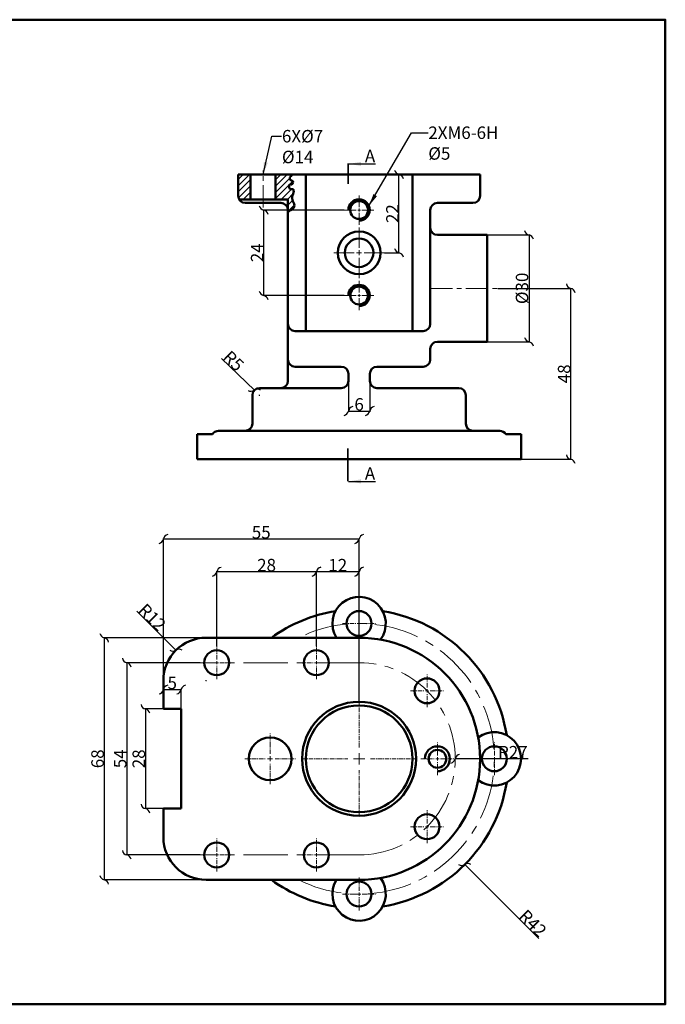
# Model space of a CAD drawing. Units: millimetres. Extents: x 10 to 373, y 9 to 285.
# Tile 3 of 3: x 191 to 373, y 9 to 285. Entities that reach past the tile are written whole.
import ezdxf

# ---------------------------------------------------------------- set-up
doc = ezdxf.new("R2010")
doc.units = ezdxf.units.MM
doc.header["$MEASUREMENT"] = 0
doc.linetypes.add('CENTER', pattern=[2, 1.25, -0.25, 0.25, -0.25])
for name, color, linetype, lineweight in [('M-CNTR', 1, 'CENTER', 18), ('M-DIMS', 2, 'Continuous', 25), ('M-HATC', 8, 'Continuous', 18), ('M-OUTL', 7, 'Continuous', 50), ('M-SECT', 7, 'Continuous', 35), ('M-TEXT', 7, 'Continuous', 25), ('M-TTLB', 7, 'Continuous', 50)]:
    doc.layers.add(name, color=color, linetype=linetype, lineweight=lineweight)
doc.styles.get("Standard").update_dxf_attribs({"font": 'arial.ttf'})
doc.dimstyles.get("Standard").update_dxf_attribs({"dimtxt": 3.5, "dimasz": 3.5, "dimexe": 0.18, "dimexo": 0.0625, "dimgap": 0.09, "dimtad": 1, "dimdec": 0, "dimzin": 0, "dimdsep": 46, "dimtxsty": 'Standard', "dimblk": 'INTEGRAL', "dimcen": 0.09, "dimclre": 251, "dimadec": 0, "dimazin": 0, "dimtfac": 1, "dimtdec": 0, "dimtofl": 0, "dimtmove": 0, "dimatfit": 3, "dimfxl": 1, "dimtolj": 1, "dimtzin": 0, "dimarcsym": 0})

# ---------------------------------------------------------------- blocks, each defined once
blk = doc.blocks.new('*U5')
at = {"layer": 'M-CNTR', "color": 0, "transparency": 16777216}
for p, q in [((0, 0.9), (0, 4.62)), ((-4.62, 0), (-0.9, 0)), ((0.9, 0), (4.62, 0)), ((0, -4.62), (0, -0.9))]:
    blk.add_line(p, q, dxfattribs=at)
at = {"layer": 'M-CNTR', "color": 0, "linetype": 'Continuous', "transparency": 16777216}
for p, q in [((-0.45, 0), (0.45, 0)), ((0, -0.45), (0, 0.45))]:
    blk.add_line(p, q, dxfattribs=at)
blk = doc.blocks.new('*U6')
at = {"layer": 'M-CNTR', "color": 0, "transparency": 16777216}
for p, q in [((0, 0.9), (0, 4.62)), ((-4.62, 0), (-0.9, 0)), ((0.9, 0), (4.62, 0)), ((0, -4.62), (0, -0.9))]:
    blk.add_line(p, q, dxfattribs=at)
at = {"layer": 'M-CNTR', "color": 0, "linetype": 'Continuous', "transparency": 16777216}
for p, q in [((-0.45, 0), (0.45, 0)), ((0, -0.45), (0, 0.45))]:
    blk.add_line(p, q, dxfattribs=at)
blk = doc.blocks.new('*U7')
at = {"layer": 'M-CNTR', "color": 0, "transparency": 16777216}
for p, q in [((0, 0.9), (0, 4.62)), ((-4.62, 0), (-0.9, 0)), ((0.9, 0), (4.62, 0)), ((0, -4.62), (0, -0.9))]:
    blk.add_line(p, q, dxfattribs=at)
at = {"layer": 'M-CNTR', "color": 0, "linetype": 'Continuous', "transparency": 16777216}
for p, q in [((-0.45, 0), (0.45, 0)), ((0, -0.45), (0, 0.45))]:
    blk.add_line(p, q, dxfattribs=at)
blk = doc.blocks.new('*U8')
at = {"layer": 'M-CNTR', "color": 0, "transparency": 16777216}
for p, q in [((0, 0.9), (0, 4.62)), ((-4.62, 0), (-0.9, 0)), ((0.9, 0), (4.62, 0)), ((0, -4.62), (0, -0.9))]:
    blk.add_line(p, q, dxfattribs=at)
at = {"layer": 'M-CNTR', "color": 0, "linetype": 'Continuous', "transparency": 16777216}
for p, q in [((-0.45, 0), (0.45, 0)), ((0, -0.45), (0, 0.45))]:
    blk.add_line(p, q, dxfattribs=at)
blk = doc.blocks.new('*U9')
at = {"layer": 'M-CNTR', "color": 0, "transparency": 16777216}
for p, q in [((0, 0.9), (0, 4.62)), ((-4.62, 0), (-0.9, 0)), ((0.9, 0), (4.62, 0)), ((0, -4.62), (0, -0.9))]:
    blk.add_line(p, q, dxfattribs=at)
at = {"layer": 'M-CNTR', "color": 0, "linetype": 'Continuous', "transparency": 16777216}
for p, q in [((-0.45, 0), (0.45, 0)), ((0, -0.45), (0, 0.45))]:
    blk.add_line(p, q, dxfattribs=at)
blk = doc.blocks.new('*U10')
at = {"layer": 'M-CNTR', "color": 0, "transparency": 16777216}
for p, q in [((0, 0.9), (0, 4.62)), ((-4.62, 0), (-0.9, 0)), ((0.9, 0), (4.62, 0)), ((0, -4.62), (0, -0.9))]:
    blk.add_line(p, q, dxfattribs=at)
at = {"layer": 'M-CNTR', "color": 0, "linetype": 'Continuous', "transparency": 16777216}
for p, q in [((-0.45, 0), (0.45, 0)), ((0, -0.45), (0, 0.45))]:
    blk.add_line(p, q, dxfattribs=at)
blk = doc.blocks.new('*U11')
at = {"layer": 'M-CNTR', "color": 0, "transparency": 16777216}
for p, q in [((0, 0.9), (0, 4.62)), ((-4.62, 0), (-0.9, 0)), ((0.9, 0), (4.62, 0)), ((0, -4.62), (0, -0.9))]:
    blk.add_line(p, q, dxfattribs=at)
at = {"layer": 'M-CNTR', "color": 0, "linetype": 'Continuous', "transparency": 16777216}
for p, q in [((-0.45, 0), (0.45, 0)), ((0, -0.45), (0, 0.45))]:
    blk.add_line(p, q, dxfattribs=at)
blk = doc.blocks.new('*U12')
at = {"layer": 'M-CNTR', "color": 0, "transparency": 16777216}
for p, q in [((0, 1.4), (0, 7.12)), ((-7.12, 0), (-1.4, 0)), ((1.4, 0), (7.12, 0)), ((0, -7.12), (0, -1.4))]:
    blk.add_line(p, q, dxfattribs=at)
at = {"layer": 'M-CNTR', "color": 0, "linetype": 'Continuous', "transparency": 16777216}
for p, q in [((-0.7, 0), (0.7, 0)), ((0, -0.7), (0, 0.7))]:
    blk.add_line(p, q, dxfattribs=at)
blk = doc.blocks.new('*U13')
at = {"layer": 'M-CNTR', "color": 0, "transparency": 16777216}
for p, q in [((0, 3.2), (0, 16.12)), ((-16.12, 0), (-3.2, 0)), ((3.2, 0), (16.12, 0)), ((0, -16.12), (0, -3.2))]:
    blk.add_line(p, q, dxfattribs=at)
at = {"layer": 'M-CNTR', "color": 0, "linetype": 'Continuous', "transparency": 16777216}
for p, q in [((-1.6, 0), (1.6, 0)), ((0, -1.6), (0, 1.6))]:
    blk.add_line(p, q, dxfattribs=at)
blk = doc.blocks.new('*U14')
at = {"layer": 'M-CNTR', "color": 0, "transparency": 16777216}
for p, q in [((0, 0.9), (0, 4.62)), ((-4.62, 0), (-0.9, 0)), ((0.9, 0), (4.62, 0)), ((0, -4.62), (0, -0.9))]:
    blk.add_line(p, q, dxfattribs=at)
at = {"layer": 'M-CNTR', "color": 0, "linetype": 'Continuous', "transparency": 16777216}
for p, q in [((-0.45, 0), (0.45, 0)), ((0, -0.45), (0, 0.45))]:
    blk.add_line(p, q, dxfattribs=at)
blk = doc.blocks.new('*U15')
at = {"layer": 'M-CNTR', "color": 0, "transparency": 16777216}
for p, q in [((0, 0.9), (0, 4.62)), ((-4.62, 0), (-0.9, 0)), ((0.9, 0), (4.62, 0)), ((0, -4.62), (0, -0.9))]:
    blk.add_line(p, q, dxfattribs=at)
at = {"layer": 'M-CNTR', "color": 0, "linetype": 'Continuous', "transparency": 16777216}
for p, q in [((-0.45, 0), (0.45, 0)), ((0, -0.45), (0, 0.45))]:
    blk.add_line(p, q, dxfattribs=at)
blk = doc.blocks.new('*U16')
at = {"layer": 'M-CNTR', "color": 0, "transparency": 16777216}
for p, q in [((0, 0.9), (0, 4.62)), ((-4.62, 0), (-0.9, 0)), ((0.9, 0), (4.62, 0)), ((0, -4.62), (0, -0.9))]:
    blk.add_line(p, q, dxfattribs=at)
at = {"layer": 'M-CNTR', "color": 0, "linetype": 'Continuous', "transparency": 16777216}
for p, q in [((-0.45, 0), (0.45, 0)), ((0, -0.45), (0, 0.45))]:
    blk.add_line(p, q, dxfattribs=at)
blk = doc.blocks.new('*U20')
at = {"layer": 'M-CNTR', "color": 0, "ltscale": 5, "transparency": 16777216}
for p, q in [((0, 0.8), (0, 4.12)), ((-4.12, 0), (-0.8, 0)), ((0.8, 0), (4.12, 0)), ((0, -4.12), (0, -0.8))]:
    blk.add_line(p, q, dxfattribs=at)
at = {"layer": 'M-CNTR', "color": 0, "linetype": 'Continuous', "ltscale": 5, "transparency": 16777216}
for p, q in [((-0.4, 0), (0.4, 0)), ((0, -0.4), (0, 0.4))]:
    blk.add_line(p, q, dxfattribs=at)
blk = doc.blocks.new('*U21')
at = {"layer": 'M-CNTR', "color": 0, "ltscale": 5, "transparency": 16777216}
for p, q in [((0, 1.4), (0, 7.12)), ((-7.12, 0), (-1.4, 0)), ((1.4, 0), (7.12, 0)), ((0, -7.12), (0, -1.4))]:
    blk.add_line(p, q, dxfattribs=at)
at = {"layer": 'M-CNTR', "color": 0, "linetype": 'Continuous', "ltscale": 5, "transparency": 16777216}
for p, q in [((-0.7, 0), (0.7, 0)), ((0, -0.7), (0, 0.7))]:
    blk.add_line(p, q, dxfattribs=at)
blk = doc.blocks.new('*U22')
at = {"layer": 'M-CNTR', "color": 0, "ltscale": 5, "transparency": 16777216}
for p, q in [((0, 0.8), (0, 4.12)), ((-4.12, 0), (-0.8, 0)), ((0.8, 0), (4.12, 0)), ((0, -4.12), (0, -0.8))]:
    blk.add_line(p, q, dxfattribs=at)
at = {"layer": 'M-CNTR', "color": 0, "linetype": 'Continuous', "ltscale": 5, "transparency": 16777216}
for p, q in [((-0.4, 0), (0.4, 0)), ((0, -0.4), (0, 0.4))]:
    blk.add_line(p, q, dxfattribs=at)
blk = doc.blocks.new('_Integral')
at = {"color": 0, "linetype": 'ByBlock', "lineweight": -2}
for centre, start, end in [((0.445, -0.091), 102, 168), ((-0.445, 0.091), 282, 348)]:
    blk.add_arc(centre, 0.454, start, end, dxfattribs=at)
blk = doc.blocks.new('*D45')
at = {"layer": 'Defpoints', "color": 0, "transparency": 16777216}
for p in [(259.92, 231.9), (282.61, 231.9), (282.61, 207.9)]:
    blk.add_point(p, dxfattribs=at)
at = {"layer": 'M-DIMS', "color": 0, "lineweight": -2, "transparency": 16777216}
for p, q in [((282.54, 231.9), (259.74, 231.9)), ((259.92, 207.9), (259.92, 231.9)), ((282.54, 207.9), (259.74, 207.9))]:
    blk.add_line(p, q, dxfattribs=at)
at = {"layer": 'M-DIMS', "color": 0, "lineweight": -2, "transparency": 16777216, "xscale": 3.5, "yscale": 3.5, "zscale": 3.5}
for p, rotation in [((259.92, 231.9), 90), ((259.92, 207.9), 270)]:
    blk.add_blockref('_Integral', p, dxfattribs=dict(at, rotation=rotation))
at = {"layer": 'M-DIMS', "color": 0, "transparency": 16777216, "insert": (258.07, 219.9), "char_height": 3.5, "attachment_point": 5, "rotation": 90}
blk.add_mtext('\\A1;24', dxfattribs=at)
blk = doc.blocks.new('*D46')
at = {"layer": 'Defpoints', "color": 0, "transparency": 16777216}
for p in [(297.94, 241.9), (298.06, 241.9), (293.85, 219.9)]:
    blk.add_point(p, dxfattribs=at)
at = {"layer": 'M-DIMS', "color": 0, "lineweight": -2, "transparency": 16777216}
for p, q in [((298, 241.9), (297.76, 241.9)), ((297.94, 219.9), (297.94, 241.9)), ((293.91, 219.9), (298.12, 219.9))]:
    blk.add_line(p, q, dxfattribs=at)
at = {"layer": 'M-DIMS', "color": 0, "lineweight": -2, "transparency": 16777216, "xscale": 3.5, "yscale": 3.5, "zscale": 3.5}
for p, rotation in [((297.94, 241.9), 90), ((297.94, 219.9), 270)]:
    blk.add_blockref('_Integral', p, dxfattribs=dict(at, rotation=rotation))
at = {"layer": 'M-DIMS', "color": 0, "transparency": 16777216, "insert": (296.09, 230.9), "char_height": 3.5, "attachment_point": 5, "rotation": 90}
blk.add_mtext('\\A1;22', dxfattribs=at)
blk = doc.blocks.new('*D47')
at = {"layer": 'Defpoints', "color": 0, "transparency": 16777216}
for p in [(322.73, 224.9), (322.73, 194.9), (334.48, 194.9)]:
    blk.add_point(p, dxfattribs=at)
at = {"layer": 'M-DIMS', "color": 0, "lineweight": -2, "transparency": 16777216}
for p, q in [((322.79, 224.9), (334.66, 224.9)), ((334.48, 224.9), (334.48, 194.9)), ((322.79, 194.9), (334.66, 194.9))]:
    blk.add_line(p, q, dxfattribs=at)
at = {"layer": 'M-DIMS', "color": 0, "lineweight": -2, "transparency": 16777216, "xscale": 3.5, "yscale": 3.5, "zscale": 3.5}
for p, rotation in [((334.48, 224.9), 90), ((334.48, 194.9), 270)]:
    blk.add_blockref('_Integral', p, dxfattribs=dict(at, rotation=rotation))
at = {"layer": 'M-DIMS', "color": 0, "transparency": 16777216, "insert": (332.51, 209.9), "char_height": 3.5, "attachment_point": 5, "rotation": 90}
blk.add_mtext('\\A1;%%C30', dxfattribs=at)
blk = doc.blocks.new('*D48')
at = {"layer": 'Defpoints', "color": 0, "transparency": 16777216}
for p in [(283.73, 183.9), (289.73, 183.9), (289.73, 175.44)]:
    blk.add_point(p, dxfattribs=at)
at = {"layer": 'M-DIMS', "color": 0, "lineweight": -2, "transparency": 16777216}
for p, q in [((283.73, 183.84), (283.73, 175.26)), ((289.73, 183.84), (289.73, 175.26)), ((283.73, 175.44), (289.73, 175.44))]:
    blk.add_line(p, q, dxfattribs=at)
at = {"layer": 'M-DIMS', "color": 0, "lineweight": -2, "transparency": 16777216, "xscale": 3.5, "yscale": 3.5, "zscale": 3.5, "rotation": 180}
blk.add_blockref('_Integral', (283.73, 175.44), dxfattribs=at)
at = {"layer": 'M-DIMS', "color": 0, "lineweight": -2, "transparency": 16777216, "xscale": 3.5, "yscale": 3.5, "zscale": 3.5}
blk.add_blockref('_Integral', (289.73, 175.44), dxfattribs=at)
at = {"layer": 'M-DIMS', "color": 0, "transparency": 16777216, "insert": (286.73, 177.32), "char_height": 3.5, "attachment_point": 5}
blk.add_mtext('\\A1;6', dxfattribs=at)
blk = doc.blocks.new('*D49')
at = {"layer": 'Defpoints', "color": 0, "transparency": 16777216}
for p in [(257.29, 181.29), (258.73, 179.9)]:
    blk.add_point(p, dxfattribs=at)
at = {"layer": 'M-DIMS', "color": 0, "lineweight": -2, "transparency": 16777216}
for p, q in [((248.05, 190.22), (257.29, 181.29)), ((258.64, 179.9), (258.82, 179.9)), ((258.73, 179.81), (258.73, 179.99))]:
    blk.add_line(p, q, dxfattribs=at)
at = {"layer": 'M-DIMS', "color": 0, "lineweight": -2, "transparency": 16777216, "xscale": 3.5, "yscale": 3.5, "zscale": 3.5, "rotation": 315.9975904098443}
blk.add_blockref('_Integral', (257.29, 181.29), dxfattribs=at)
at = {"layer": 'M-DIMS', "color": 0, "transparency": 16777216, "insert": (251.45, 189.53), "char_height": 3.5, "attachment_point": 5, "rotation": 315.9976}
blk.add_mtext('\\A1;R5', dxfattribs=at)
blk = doc.blocks.new('*D50')
at = {"layer": 'Defpoints', "color": 0, "transparency": 16777216}
for p in [(274.73, 130.31), (274.73, 109.38), (286.73, 93.76)]:
    blk.add_point(p, dxfattribs=at)
at = {"layer": 'M-DIMS', "color": 0, "lineweight": -2, "transparency": 16777216}
for p, q in [((274.73, 109.44), (274.73, 130.49)), ((286.73, 130.31), (274.73, 130.31)), ((286.73, 93.82), (286.73, 130.49))]:
    blk.add_line(p, q, dxfattribs=at)
at = {"layer": 'M-DIMS', "color": 0, "lineweight": -2, "transparency": 16777216, "xscale": 3.5, "yscale": 3.5, "zscale": 3.5, "rotation": 180}
blk.add_blockref('_Integral', (274.73, 130.31), dxfattribs=at)
at = {"layer": 'M-DIMS', "color": 0, "lineweight": -2, "transparency": 16777216, "xscale": 3.5, "yscale": 3.5, "zscale": 3.5}
blk.add_blockref('_Integral', (286.73, 130.31), dxfattribs=at)
at = {"layer": 'M-DIMS', "color": 0, "transparency": 16777216, "insert": (280.73, 132.15), "char_height": 3.5, "attachment_point": 5}
blk.add_mtext('\\A1;12', dxfattribs=at)
blk = doc.blocks.new('*D51')
at = {"layer": 'Defpoints', "color": 0, "transparency": 16777216}
for p in [(246.73, 130.3), (246.73, 109.38), (274.73, 109.38)]:
    blk.add_point(p, dxfattribs=at)
at = {"layer": 'M-DIMS', "color": 0, "lineweight": -2, "transparency": 16777216}
for p, q in [((246.73, 109.44), (246.73, 130.48)), ((274.73, 130.3), (246.73, 130.3)), ((274.73, 109.44), (274.73, 130.48))]:
    blk.add_line(p, q, dxfattribs=at)
at = {"layer": 'M-DIMS', "color": 0, "lineweight": -2, "transparency": 16777216, "xscale": 3.5, "yscale": 3.5, "zscale": 3.5, "rotation": 180}
blk.add_blockref('_Integral', (246.73, 130.3), dxfattribs=at)
at = {"layer": 'M-DIMS', "color": 0, "lineweight": -2, "transparency": 16777216, "xscale": 3.5, "yscale": 3.5, "zscale": 3.5}
blk.add_blockref('_Integral', (274.73, 130.3), dxfattribs=at)
at = {"layer": 'M-DIMS', "color": 0, "transparency": 16777216, "insert": (260.73, 132.17), "char_height": 3.5, "attachment_point": 5}
blk.add_mtext('\\A1;28', dxfattribs=at)
blk = doc.blocks.new('*D52')
at = {"layer": 'Defpoints', "color": 0, "transparency": 16777216}
for p in [(231.73, 139.49), (231.73, 99.76), (286.73, 93.88)]:
    blk.add_point(p, dxfattribs=at)
at = {"layer": 'M-DIMS', "color": 0, "lineweight": -2, "transparency": 16777216}
for p, q in [((231.73, 99.82), (231.73, 139.67)), ((286.73, 139.49), (231.73, 139.49)), ((286.73, 93.94), (286.73, 139.67))]:
    blk.add_line(p, q, dxfattribs=at)
at = {"layer": 'M-DIMS', "color": 0, "lineweight": -2, "transparency": 16777216, "xscale": 3.5, "yscale": 3.5, "zscale": 3.5, "rotation": 180}
blk.add_blockref('_Integral', (231.73, 139.49), dxfattribs=at)
at = {"layer": 'M-DIMS', "color": 0, "lineweight": -2, "transparency": 16777216, "xscale": 3.5, "yscale": 3.5, "zscale": 3.5}
blk.add_blockref('_Integral', (286.73, 139.49), dxfattribs=at)
at = {"layer": 'M-DIMS', "color": 0, "transparency": 16777216, "insert": (259.23, 141.36), "char_height": 3.5, "attachment_point": 5}
blk.add_mtext('\\A1;55', dxfattribs=at)
blk = doc.blocks.new('*D53')
at = {"layer": 'Defpoints', "color": 0, "transparency": 16777216}
for p in [(243.73, 111.76), (215.11, 43.76), (243.73, 43.76)]:
    blk.add_point(p, dxfattribs=at)
at = {"layer": 'M-DIMS', "color": 0, "lineweight": -2, "transparency": 16777216}
for p, q in [((243.66, 111.76), (214.93, 111.76)), ((215.11, 111.76), (215.11, 43.76)), ((243.66, 43.76), (214.93, 43.76))]:
    blk.add_line(p, q, dxfattribs=at)
at = {"layer": 'M-DIMS', "color": 0, "lineweight": -2, "transparency": 16777216, "xscale": 3.5, "yscale": 3.5, "zscale": 3.5}
for p, rotation in [((215.11, 111.76), 90), ((215.11, 43.76), 270)]:
    blk.add_blockref('_Integral', p, dxfattribs=dict(at, rotation=rotation))
at = {"layer": 'M-DIMS', "color": 0, "transparency": 16777216, "insert": (213.23, 77.76), "char_height": 3.5, "attachment_point": 5, "rotation": 90}
blk.add_mtext('\\A1;68', dxfattribs=at)
blk = doc.blocks.new('*D54')
at = {"layer": 'Defpoints', "color": 0, "transparency": 16777216}
for p in [(242.11, 104.76), (221.45, 50.76), (242.11, 50.76)]:
    blk.add_point(p, dxfattribs=at)
at = {"layer": 'M-DIMS', "color": 0, "lineweight": -2, "transparency": 16777216}
for p, q in [((242.04, 104.76), (221.27, 104.76)), ((221.45, 104.76), (221.45, 50.76)), ((242.04, 50.76), (221.27, 50.76))]:
    blk.add_line(p, q, dxfattribs=at)
at = {"layer": 'M-DIMS', "color": 0, "lineweight": -2, "transparency": 16777216, "xscale": 3.5, "yscale": 3.5, "zscale": 3.5}
for p, rotation in [((221.45, 104.76), 90), ((221.45, 50.76), 270)]:
    blk.add_blockref('_Integral', p, dxfattribs=dict(at, rotation=rotation))
at = {"layer": 'M-DIMS', "color": 0, "transparency": 16777216, "insert": (219.58, 77.76), "char_height": 3.5, "attachment_point": 5, "rotation": 90}
blk.add_mtext('\\A1;54', dxfattribs=at)
blk = doc.blocks.new('*D55')
at = {"layer": 'Defpoints', "color": 0, "transparency": 16777216}
for p in [(231.73, 91.76), (226.69, 63.76), (231.73, 63.76)]:
    blk.add_point(p, dxfattribs=at)
at = {"layer": 'M-DIMS', "color": 0, "lineweight": -2, "transparency": 16777216}
for p, q in [((231.66, 91.76), (226.51, 91.76)), ((226.69, 91.76), (226.69, 63.76)), ((231.66, 63.76), (226.51, 63.76))]:
    blk.add_line(p, q, dxfattribs=at)
at = {"layer": 'M-DIMS', "color": 0, "lineweight": -2, "transparency": 16777216, "xscale": 3.5, "yscale": 3.5, "zscale": 3.5}
for p, rotation in [((226.69, 91.76), 90), ((226.69, 63.76), 270)]:
    blk.add_blockref('_Integral', p, dxfattribs=dict(at, rotation=rotation))
at = {"layer": 'M-DIMS', "color": 0, "transparency": 16777216, "insert": (224.81, 77.76), "char_height": 3.5, "attachment_point": 5, "rotation": 90}
blk.add_mtext('\\A1;28', dxfattribs=at)
blk = doc.blocks.new('*D56')
at = {"layer": 'Defpoints', "color": 0, "transparency": 16777216}
for p in [(231.73, 97.21), (236.73, 97.21), (236.73, 91.76)]:
    blk.add_point(p, dxfattribs=at)
at = {"layer": 'M-DIMS', "color": 0, "lineweight": -2, "transparency": 16777216}
for p, q in [((231.73, 97.27), (231.73, 97.39)), ((231.73, 97.21), (236.73, 97.21)), ((236.73, 91.82), (236.73, 97.39))]:
    blk.add_line(p, q, dxfattribs=at)
at = {"layer": 'M-DIMS', "color": 0, "lineweight": -2, "transparency": 16777216, "xscale": 3.5, "yscale": 3.5, "zscale": 3.5, "rotation": 180}
blk.add_blockref('_Integral', (231.73, 97.21), dxfattribs=at)
at = {"layer": 'M-DIMS', "color": 0, "lineweight": -2, "transparency": 16777216, "xscale": 3.5, "yscale": 3.5, "zscale": 3.5}
blk.add_blockref('_Integral', (236.73, 97.21), dxfattribs=at)
at = {"layer": 'M-DIMS', "color": 0, "transparency": 16777216, "insert": (234.23, 99.08), "char_height": 3.5, "attachment_point": 5}
blk.add_mtext('\\A1;5', dxfattribs=at)
blk = doc.blocks.new('*D65')
at = {"layer": 'Defpoints', "color": 0, "transparency": 16777216}
for p in [(325.68, 209.9), (346.21, 209.9), (332.23, 161.9)]:
    blk.add_point(p, dxfattribs=at)
at = {"layer": 'M-DIMS', "color": 0, "lineweight": -2, "transparency": 16777216}
for p, q in [((325.74, 209.9), (346.39, 209.9)), ((346.21, 161.9), (346.21, 209.9)), ((332.29, 161.9), (346.39, 161.9))]:
    blk.add_line(p, q, dxfattribs=at)
at = {"layer": 'M-DIMS', "color": 0, "lineweight": -2, "transparency": 16777216, "xscale": 3.5, "yscale": 3.5, "zscale": 3.5}
for p, rotation in [((346.21, 209.9), 90), ((346.21, 161.9), 270)]:
    blk.add_blockref('_Integral', p, dxfattribs=dict(at, rotation=rotation))
at = {"layer": 'M-DIMS', "color": 0, "transparency": 16777216, "insert": (344.33, 185.9), "char_height": 3.5, "attachment_point": 5, "rotation": 90}
blk.add_mtext('\\A1;48', dxfattribs=at)
blk = doc.blocks.new('*D67')
at = {"layer": 'Defpoints', "color": 0, "transparency": 16777216}
for p in [(286.73, 77.76), (316.43, 48.07)]:
    blk.add_point(p, dxfattribs=at)
at = {"layer": 'M-DIMS', "color": 251, "lineweight": -2, "transparency": 16777216}
for p, q in [((286.64, 77.76), (286.82, 77.76)), ((286.73, 77.67), (286.73, 77.85))]:
    blk.add_line(p, q, dxfattribs=at)
at = {"layer": 'M-DIMS', "color": 0, "lineweight": -2, "transparency": 16777216}
blk.add_line((337.26, 27.25), (316.43, 48.07), dxfattribs=at)
at = {"layer": 'M-DIMS', "color": 0, "lineweight": -2, "transparency": 16777216, "xscale": 3.5, "yscale": 3.5, "zscale": 3.5, "rotation": 135.0109880390771}
blk.add_blockref('_Integral', (316.43, 48.07), dxfattribs=at)
at = {"layer": 'M-DIMS', "color": 0, "transparency": 16777216, "insert": (335.56, 31.56), "char_height": 3.5, "attachment_point": 5, "rotation": 315.011}
blk.add_mtext('\\A1;R42', dxfattribs=at)
blk = doc.blocks.new('*D69')
at = {"layer": 'Defpoints', "color": 0, "transparency": 16777216}
for p in [(235.24, 108.25), (243.73, 99.76)]:
    blk.add_point(p, dxfattribs=at)
at = {"layer": 'M-DIMS', "color": 0, "lineweight": -2, "transparency": 16777216}
blk.add_line((224.28, 119.21), (235.24, 108.25), dxfattribs=at)
at = {"layer": 'M-DIMS', "color": 251, "lineweight": -2, "transparency": 16777216}
for p, q in [((243.64, 99.76), (243.82, 99.76)), ((243.73, 99.67), (243.73, 99.85))]:
    blk.add_line(p, q, dxfattribs=at)
at = {"layer": 'M-DIMS', "color": 0, "lineweight": -2, "transparency": 16777216, "xscale": 3.5, "yscale": 3.5, "zscale": 3.5, "rotation": 314.9987204254547}
blk.add_blockref('_Integral', (235.24, 108.25), dxfattribs=at)
at = {"layer": 'M-DIMS', "color": 0, "transparency": 16777216, "insert": (228.59, 117.51), "char_height": 3.5, "attachment_point": 5, "rotation": 314.9987}
blk.add_mtext('\\A1;R12', dxfattribs=at)
blk = doc.blocks.new('*D70')
at = {"layer": 'Defpoints', "color": 0, "transparency": 16777216}
for p in [(286.73, 77.76), (313.73, 77.76)]:
    blk.add_point(p, dxfattribs=at)
at = {"layer": 'M-DIMS', "color": 251, "lineweight": -2, "transparency": 16777216}
for p, q in [((286.64, 77.76), (286.82, 77.76)), ((286.73, 77.67), (286.73, 77.85))]:
    blk.add_line(p, q, dxfattribs=at)
at = {"layer": 'M-DIMS', "color": 0, "lineweight": -2, "transparency": 16777216}
blk.add_line((334.2, 77.76), (313.73, 77.76), dxfattribs=at)
at = {"layer": 'M-DIMS', "color": 0, "lineweight": -2, "transparency": 16777216, "xscale": 3.5, "yscale": 3.5, "zscale": 3.5, "rotation": 180.0009315869335}
blk.add_blockref('_Integral', (313.73, 77.76), dxfattribs=at)
at = {"layer": 'M-DIMS', "color": 0, "transparency": 16777216, "insert": (329.93, 79.61), "char_height": 3.5, "attachment_point": 5, "rotation": 0.0009}
blk.add_mtext('\\A1;R27', dxfattribs=at)

msp = doc.modelspace()

# ---------------------------------------------------------------- hatches: boundary and pattern name
at = {"layer": 'M-HATC'}
h = msp.add_hatch(dxfattribs=at)
h.set_pattern_fill('ANSI31', color=256, scale=10)
h.set_pattern_definition([(45, (-376.4816, -107.6296), (-0.8838835, 0.8838835), [])])
h.paths.add_polyline_path([(252.73, 235.9, 0.131652), (253, 234.9), (256.23, 234.9), (256.23, 241.9), (252.73, 241.9)])
edge = h.paths.add_edge_path()
edge.add_spline(control_points=[(266.73, 231.45), (267.06, 231.65), (268.96, 232.47), (268.31, 234.01), (267.68, 235.4), (268.34, 236.4), (268.51, 238.02), (267.13, 237.41), (266.77, 239.27), (267.99, 238.89), (268.4, 240.18), (266.79, 240.3), (267.4, 241.27), (267.8, 241.9)], knot_values=[0, 0, 0, 0, 1.296255, 2.906349, 4.421341, 5.455336, 6.72765, 7.411554, 8.713533, 9.35604, 10.281891, 11.112123, 12.701769, 12.701769, 12.701769, 12.701769], degree=3, periodic=0)
edge.add_line((267.8, 241.9), (263.23, 241.9))
edge.add_line((263.23, 241.9), (263.23, 234.9))
edge.add_line((263.23, 234.9), (266.73, 234.9))
edge.add_line((266.73, 234.9), (266.73, 231.45))

# ---------------------------------------------------------------- linework, layer by layer
at = {"layer": 'M-CNTR', "ltscale": 5}
for p, q in [((259.73, 232.62), (259.73, 242.96)), ((306.73, 209.9), (325.68, 209.9))]:
    msp.add_line(p, q, dxfattribs=at)
at = {"layer": 'M-CNTR', "ltscale": 10}
for p, q in [((286.73, 104.76), (232.82, 104.76)), ((286.73, 50.76), (232.82, 50.76))]:
    msp.add_line(p, q, dxfattribs=at)
for radius, start, end in [(38, 243.4746, 116.5254), (27, 270, 90)]:
    msp.add_arc((286.73, 77.76), radius, start, end, dxfattribs=at)
at = {"layer": 'M-OUTL'}
for p, q in [((252.73, 241.9), (320.73, 241.9)), ((252.73, 235.9), (252.73, 241.9)), ((256.23, 234.9), (256.23, 241.9)), ((263.23, 234.9), (263.23, 241.9)), ((271.73, 241.9), (271.73, 197.9)), ((301.73, 241.9), (301.73, 197.9)), ((320.73, 241.9), (320.73, 235.9)), ((253, 234.9), (266.73, 234.9)), ((254.73, 233.9), (264.73, 233.9)), ((266.73, 189.9), (266.73, 234.9)), ((308.73, 233.9), (318.73, 233.9)), ((306.73, 199.9), (306.73, 231.9)), ((308.73, 224.9), (322.73, 224.9)), ((322.73, 224.9), (322.73, 194.9)), ((268.73, 197.9), (304.73, 197.9)), ((308.73, 194.9), (322.73, 194.9)), ((306.73, 189.9), (306.73, 192.9)), ((266.73, 189.9), (266.73, 183.9)), ((268.73, 187.9), (281.73, 187.9)), ((283.73, 183.9), (283.73, 185.9)), ((289.73, 183.9), (289.73, 185.9)), ((304.73, 187.9), (291.73, 187.9)), ((256.73, 171.9), (256.73, 179.9)), ((281.73, 181.9), (258.73, 181.9)), ((291.73, 181.9), (314.73, 181.9)), ((316.73, 171.9), (316.73, 179.9)), ((241.23, 168.9), (245.5, 168.9)), ((241.23, 161.9), (241.23, 168.9)), ((247.23, 169.9), (326.23, 169.9)), ((327.96, 168.9), (332.23, 168.9)), ((332.23, 161.9), (332.23, 168.9)), ((241.23, 161.9), (332.23, 161.9)), ((243.73, 111.76), (286.73, 111.76)), ((231.73, 99.76), (231.73, 91.76)), ((236.73, 91.76), (231.73, 91.76)), ((236.73, 91.76), (236.73, 63.76)), ((236.73, 63.76), (231.73, 63.76)), ((231.73, 63.76), (231.73, 55.76)), ((243.73, 43.76), (286.73, 43.76))]:
    msp.add_line(p, q, dxfattribs=at)
for centre, radius in [((286.73, 231.9), 2.5), ((286.73, 219.9), 6), ((286.73, 219.9), 4), ((286.73, 207.9), 2.5), ((286.73, 115.76), 3.5), ((246.73, 104.76), 3.5), ((274.73, 104.76), 3.5), ((305.82, 96.85), 3.5), ((286.73, 77.76), 16), ((286.73, 77.76), 15), ((261.73, 77.76), 6), ((308.73, 77.76), 2.5), ((324.73, 77.76), 3.5), ((305.82, 58.67), 3.5), ((246.73, 50.76), 3.5), ((274.73, 50.76), 3.5), ((286.73, 39.76), 3.5)]:
    msp.add_circle(centre, radius, dxfattribs=at)
for centre, radius, start, end in [((254.73, 235.9), 2, 180, 270), ((318.73, 235.9), 2, 270, 0), ((264.73, 231.9), 2, 0, 90), ((286.73, 231.9), 3, 270, 180), ((308.73, 231.9), 2, 90, 180), ((308.73, 226.9), 2, 180, 270), ((286.73, 207.9), 3, 270, 180), ((268.73, 199.9), 2, 180, 270), ((304.73, 199.9), 2, 270, 0), ((308.73, 192.9), 2, 90, 180), ((268.73, 189.9), 2, 180, 270), ((304.73, 189.9), 2, 270, 0), ((281.73, 185.9), 2, 0, 90), ((291.73, 185.9), 2, 90, 180), ((264.73, 183.9), 2, 270, 0), ((281.73, 183.9), 2, 270, 0), ((291.73, 183.9), 2, 180, 270), ((258.73, 179.9), 2, 90, 180), ((314.73, 179.9), 2, 0, 90), ((254.73, 171.9), 2, 270, 0), ((318.73, 171.9), 2, 180, 270), ((247.23, 167.9), 2, 90, 150), ((326.23, 167.9), 2, 30, 90), ((286.73, 115.76), 7.5, 322.8469, 212.231), ((286.73, 77.76), 42, 99.1085, 125.9506), ((286.73, 77.76), 42, 9.1085, 80.8915), ((243.73, 99.76), 12, 90, 180), ((286.73, 77.76), 34, 270, 90), ((324.73, 77.76), 7.5, 232.8469, 127.1531), ((308.73, 77.76), 3.5, 270, 180), ((286.73, 77.76), 42, 279.1085, 350.8915), ((243.73, 55.76), 12, 180, 270), ((286.73, 39.76), 7.5, 147.769, 37.1531), ((286.73, 77.76), 42, 234.0494, 260.8915)]:
    msp.add_arc(centre, radius, start, end, dxfattribs=at)
msp.add_open_spline([(267.8, 241.9), (267.4, 241.27), (266.79, 240.3), (268.4, 240.18), (267.99, 238.89), (266.77, 239.27), (267.13, 237.41), (268.51, 238.02), (268.34, 236.4), (267.68, 235.4), (268.31, 234.01), (268.96, 232.47), (267.06, 231.65), (266.73, 231.45)], degree=3, knots=[0, 0, 0, 0, 1.589647, 2.419879, 3.34573, 3.988237, 5.290216, 5.974119, 7.246434, 8.280428, 9.795421, 11.405514, 12.701769, 12.701769, 12.701769, 12.701769], dxfattribs=at)
at = {"layer": 'M-SECT'}
for p, q in [((283.68, 244.94), (283.68, 239.26)), ((283.6, 155.72), (283.6, 164.9))]:
    msp.add_line(p, q, dxfattribs=at)
at = {"layer": 'M-TTLB'}
msp.add_lwpolyline([(9.93, 285.37), (372.77, 285.37), (372.77, 8.8), (9.93, 8.8)], close=True, dxfattribs=at)

# ---------------------------------------------------------------- block references
at = {"layer": 'M-CNTR', "ltscale": 5}
for name, p in [('*U22', (286.73, 231.9)), ('*U21', (286.73, 219.9)), ('*U20', (286.73, 207.9))]:
    msp.add_blockref(name, p, dxfattribs=at)
at = {"layer": 'M-CNTR'}
for name, p in [('*U16', (286.73, 115.76)), ('*U5', (246.73, 104.76)), ('*U6', (274.73, 104.76)), ('*U7', (305.82, 96.85)), ('*U13', (286.73, 77.76)), ('*U12', (261.73, 77.76)), ('*U8', (308.73, 77.76)), ('*U15', (324.73, 77.76)), ('*U9', (305.82, 58.67)), ('*U11', (246.73, 50.76)), ('*U10', (274.73, 50.76)), ('*U14', (286.73, 39.76))]:
    msp.add_blockref(name, p, dxfattribs=at)

# ---------------------------------------------------------------- texts
at = {"layer": 'M-TEXT', "char_height": 3.5}
for s, insert, attachment_point in [('6X%%C7\\P%%C14', (265.05, 254.39), 1), ('2XM6-6H\\P%%C5', (306.18, 255.37), 1), ('\\A1;A', (289.8, 247.08), 5), ('\\A1;A', (289.8, 157.9), 5)]:
    msp.add_mtext(s, dxfattribs=dict(at, insert=insert, attachment_point=attachment_point))

# ---------------------------------------------------------------- dimensions: what is measured, and where the dimension line sits
at = {"layer": 'M-DIMS'}
for base, p1, p2, picture, middle in [((297.94, 241.9), (293.85, 219.9), (298.06, 241.9), '*D46', (296.09, 230.9)), ((259.92, 231.9), (282.61, 207.9), (282.61, 231.9), '*D45', (258.07, 219.9)), ((346.21, 209.9), (332.23, 161.9), (325.68, 209.9), '*D65', (344.33, 185.9)), ((215.11, 43.76), (243.73, 111.76), (243.73, 43.76), '*D53', (213.23, 77.76)), ((221.45, 50.76), (242.11, 104.76), (242.11, 50.76), '*D54', (219.58, 77.76)), ((226.69, 63.76), (231.73, 91.76), (231.73, 63.76), '*D55', (224.81, 77.76))]:
    dim = msp.add_linear_dim(base=base, p1=p1, p2=p2, angle=90, dimstyle='Standard', override={"dimclrd": 0, "dimclre": 0, "dimclrt": 0}, dxfattribs=at)
    dim.commit()
    dim.dimension.update_dxf_attribs({"geometry": picture, "text_midpoint": middle})
dim = msp.add_linear_dim(base=(334.48, 194.9), p1=(322.73, 224.9), p2=(322.73, 194.9), angle=90, text='%%C<>', dimstyle='Standard', override={"dimclrd": 0, "dimclre": 0, "dimclrt": 0}, dxfattribs=at)
dim.commit()
dim.dimension.update_dxf_attribs({"geometry": '*D47', "text_midpoint": (332.51, 209.9)})
dim = msp.add_radius_dim(center=(258.73, 179.9), mpoint=(257.29, 181.29), text='R5', dimstyle='Standard', override={"dimclrd": 0, "dimclre": 0, "dimclrt": 0}, dxfattribs=at)
dim.commit()
dim.dimension.update_dxf_attribs({"geometry": '*D49', "text_midpoint": (251.45, 189.53)})
for base, p1, p2, picture, middle in [((289.73, 175.44), (283.73, 183.9), (289.73, 183.9), '*D48', (286.73, 177.32)), ((231.73, 139.49), (286.73, 93.88), (231.73, 99.76), '*D52', (259.23, 141.36)), ((246.73, 130.3), (274.73, 109.38), (246.73, 109.38), '*D51', (260.73, 132.17)), ((274.73, 130.31), (286.73, 93.76), (274.73, 109.38), '*D50', (280.73, 132.15)), ((236.73, 97.21), (231.73, 97.21), (236.73, 91.76), '*D56', (234.23, 99.08))]:
    dim = msp.add_linear_dim(base=base, p1=p1, p2=p2, dimstyle='Standard', override={"dimclrd": 0, "dimclre": 0, "dimclrt": 0}, dxfattribs=at)
    dim.commit()
    dim.dimension.update_dxf_attribs({"geometry": picture, "text_midpoint": middle})
dim = msp.add_radius_dim(center=(243.73, 99.76), mpoint=(235.24, 108.25), dimstyle='Standard', override={"dimdec": 0, "dimlfac": 1, "dimrnd": 0, "dimzin": 0, "dimdsep": 46, "dimlunit": 2}, dxfattribs=at)
dim.commit()
dim.dimension.update_dxf_attribs({"geometry": '*D69', "text_midpoint": (228.59, 117.51)})
for mpoint, picture, middle in [((313.73, 77.76), '*D70', (329.93, 77.76)), ((316.43, 48.07), '*D67', (334.25, 30.25))]:
    dim = msp.add_radius_dim(center=(286.73, 77.76), mpoint=mpoint, dimstyle='Standard', override={"dimdec": 0, "dimlfac": 1, "dimrnd": 0, "dimzin": 0, "dimdsep": 46, "dimlunit": 2}, dxfattribs=at)
    dim.commit()
    dim.dimension.update_dxf_attribs({"geometry": picture, "text_midpoint": middle, "dimtype": 164})

# ---------------------------------------------------------------- leaders
at = {"layer": 'M-DIMS', "annotation_type": 0, "has_hookline": 1, "hookline_direction": 1}
for points, text_width in [([(259.73, 241.9), (262.24, 252.64), (264.96, 252.64)], 12.1), ([(289.49, 233.07), (301.48, 253.62), (306.09, 253.62)], 20.11)]:
    msp.add_leader(points, dimstyle='Standard', override={"dimgap": 0.09, "dimtad": 0}, dxfattribs=dict(at, text_width=text_width))
at = {"layer": 'M-DIMS'}
for points in [[(283.76, 244.86), (291.36, 244.86)], [(283.76, 155.68), (291.36, 155.68)]]:
    msp.add_leader(points, dimstyle='Standard', override={"dimgap": 0.09, "dimtad": 0}, dxfattribs=at)

doc.saveas('drawing.dxf')
